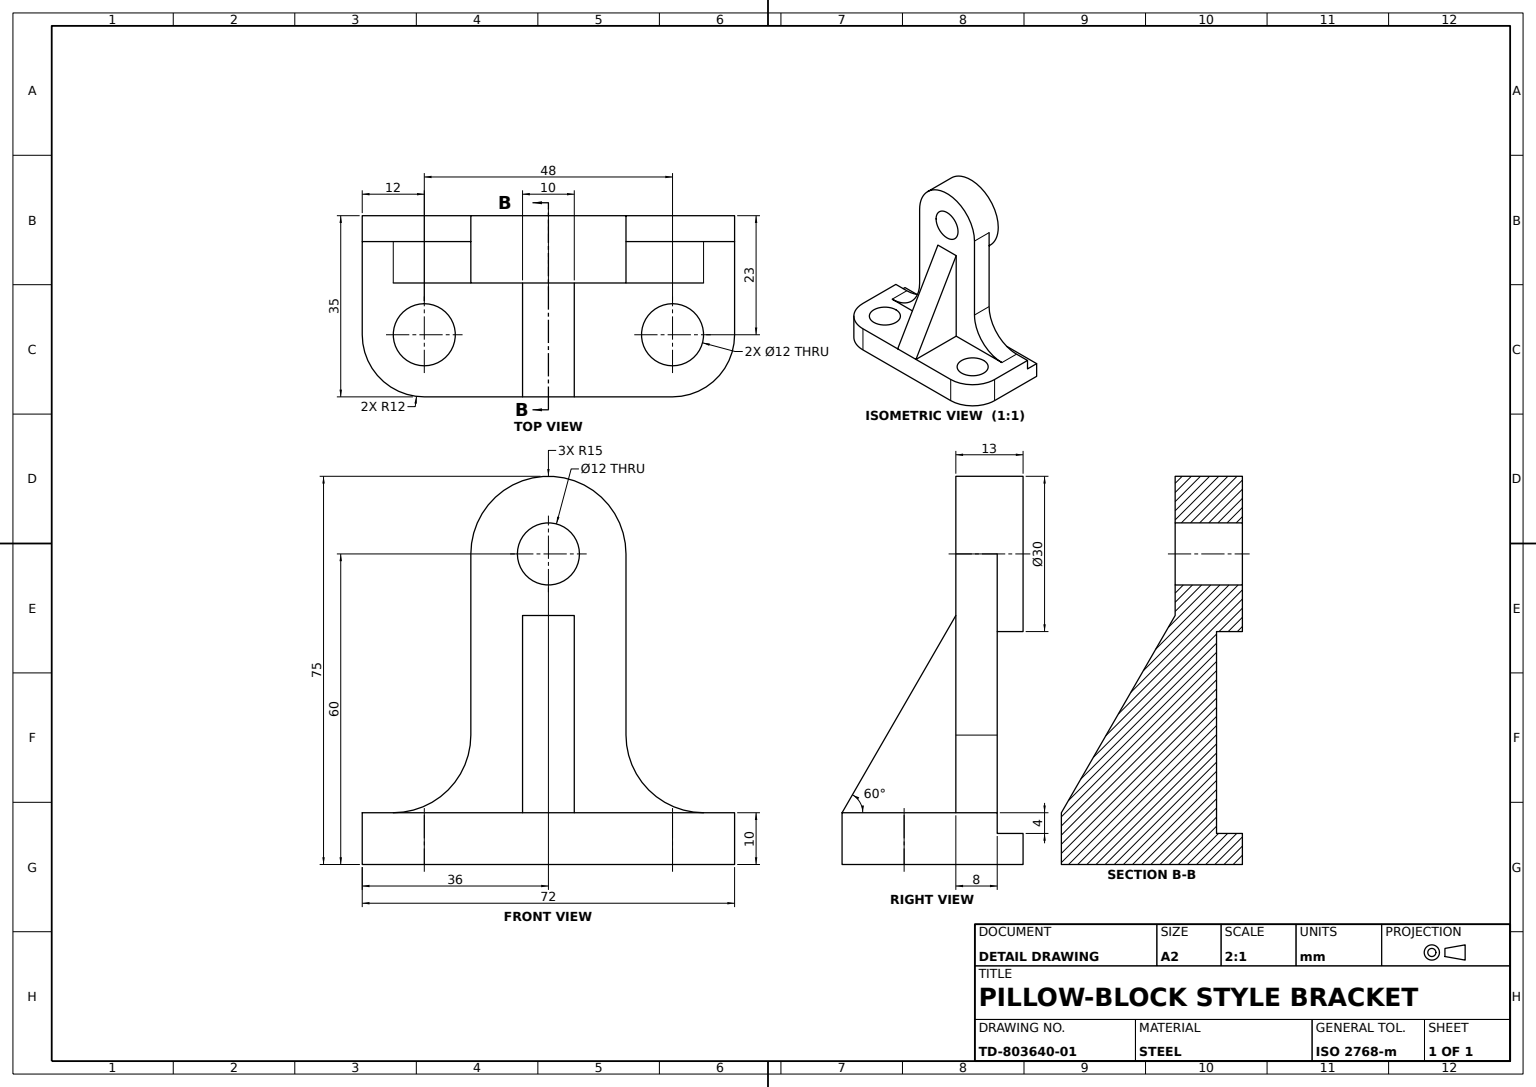
SolidWorks part; units mm, degrees
material "Plain Carbon Steel"
ref_plane "Front Plane" through (0, 0, 0) normal (0, 0, 1) x (1, 0, 0)
ref_plane "Top Plane" through (0, 0, 0) normal (0, 1, 0) x (1, 0, 0)
ref_plane "Right Plane" through (0, 0, 0) normal (1, 0, 0) x (0, 0, -1)
sketch "Base Plate Sketch" plane through (0, 0, 0) normal (0, 1, 0) x (1, 0, 0)
  line L0 (-55.2901, 0) -> (60.0819, 0) construction
  line L1 (0, -44.785) -> (0, 47.7338) construction
  line L2 (-36, 23) -> (-36, 0)
  line L3 (-36, 23) -> (36, 23)
  line L4 (36, 23) -> (36, 0)
  line L5 (-24, -12) -> (24, -12)
  circle A0 centre (-24, 0) radius 6
  circle A1 centre (24, 0) radius 6
  arc A2 (-24, -12) -> (-36, 0) centre (-24, 0) cw
  arc A3 (36, 0) -> (24, -12) centre (24, 0) cw
  point P16 (0, -12)
  dimension "D4" = 12
  dimension "D1" = 36
  dimension "D2" = 36
  dimension "D3" = 23
  dimension "D5" = 48
  dimension "D6" = 48
  dimension "D7" = 35
extrude "Base Plate" add sketch "Base Plate Sketch" along normal blind 10
sketch "Rear Groove Sketch" plane through (36, 0, 0) normal (1, 0, 0) x (0, 0, -1)
  line L0 (18, 10) -> (18, 6)
  line L1 (0, 10) -> (23, 10) construction
  line L2 (18, 6) -> (23, 6)
  line L3 (23, 10) -> (23, 0) construction
  line L4 (18, 10) -> (23, 10)
  line L5 (23, 10) -> (23, 6)
  dimension "D1" = 4
  dimension "D2" = 5
extrude "Rear Groove 4x5" cut sketch "Rear Groove Sketch" against normal through all
ref_plane "Upright Plane" through (0, 0, -18) normal (0, 0, 1) x (1, 0, 0)
sketch "Upright Sketch" plane through (0, 0, -18) normal (0, 0, 1) x (1, 0, 0)
  line L0 (0, -8.2441) -> (0, 52.2968) construction
  line L1 (-15, 10) -> (-15, 60)
  line L2 (-24, 10) -> (24, 10) construction
  line L3 (-15, 60) -> (15, 60)
  line L4 (15, 60) -> (15, 10)
  line L5 (15, 10) -> (-15, 10)
  line L6 (24, 0) -> (36, 0) construction
  dimension "D1" = 15
  dimension "60" = 60
  dimension "D2" = 15
extrude "Upright" add sketch "Upright Sketch" along normal blind 8
sketch "Hub Boss Sketch" plane through (0, 0, -10) normal (0, 0, 1) x (1, 0, 0)
  line L0 (15, 60) -> (-15, 60) construction
  circle A0 centre (0, 60) radius 15
  circle A1 centre (0, 60) radius 6
  dimension "D1" = 12
extrude "Hub Boss" add sketch "Hub Boss Sketch" against normal blind 13
sketch "Shaft Bore Sketch" plane through (0, 0, -23) normal (0, 0, -1) x (-1, 0, 0)
  circle A0 centre (0, 60) radius 6 construction
  circle A1 centre (0, 60) radius 6
extrude "Shaft Bore" cut sketch "Shaft Bore Sketch" against normal blind 13
fillet "Upright Base Fillet R15" radius 15 2 edges at (15, 10, -14) (-15, 10, -14)
sketch "Support Rib Sketch" plane through (0, 0, 0) normal (1, 0, 0) x (0, 0, -1)
  line L0 (-12, 10) -> (10, 48.1051)
  line L1 (10, 25) -> (10, 60) construction
  line L2 (0, 10) -> (-12, 10) construction
  dimension "D1" = 60
rib "Support Rib" sketch "Support Rib Sketch" sketch "Support Rib Sketch" thickness 10 extrusion direction parallel to sketch draft on no parameters "D1"=10
